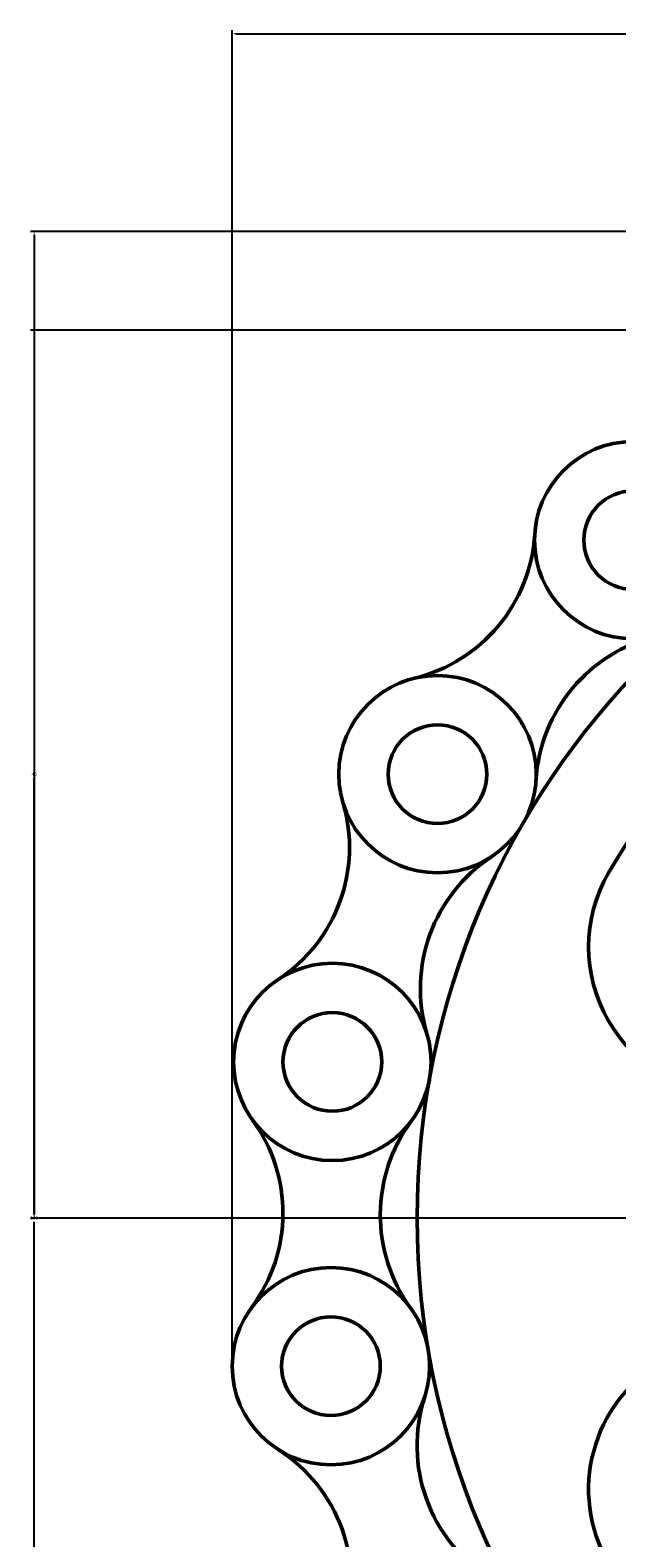
# Model space of a CAD drawing. Units: inches. Extents: x 413 to 622, y 326 to 447.
# Tile 2 of 15: x 413 to 443, y 370 to 447. Entities that reach past the tile are written whole.
import ezdxf

# ---------------------------------------------------------------- set-up
doc = ezdxf.new("R2010")
doc.units = ezdxf.units.IN
doc.header["$MEASUREMENT"] = 0
doc.layers.add('M-DIMS', color=2, linetype='Continuous', lineweight=18)
doc.layers.add('M-OUTL', color=7, linetype='Continuous', lineweight=50)
doc.styles.get("Standard").update_dxf_attribs({"font": 'arial.ttf'})
doc.dimstyles.get("Standard").update_dxf_attribs({"dimtxt": 0.18, "dimasz": 0.18, "dimexe": 0.18, "dimexo": 0.0625, "dimgap": 0.09, "dimtad": 0, "dimtih": 1, "dimtoh": 1, "dimdec": 4, "dimzin": 0, "dimdsep": 46, "dimtxsty": 'Standard', "dimcen": 0.09, "dimadec": 0, "dimazin": 0, "dimtfac": 1, "dimtdec": 4, "dimtofl": 0, "dimtmove": 0, "dimatfit": 3, "dimfxl": 1, "dimtolj": 1, "dimtzin": 0, "dimarcsym": 0})

# ---------------------------------------------------------------- blocks, each defined once
blk = doc.blocks.new('CHAIN-ROLLER-PIN')
for radius in [5, 2.5]:
    blk.add_circle((5, 5), radius)
blk = doc.blocks.new('SPROCKET-WEB-SLOT')
for centre, radius, start, end in [((7.501, 21.25), 7.5, 30, 210), ((31.317, 35), 20, 210, 270), ((31.317, 35), 35, 210, 270), ((31.317, 7.5), 7.5, 270, 90)]:
    blk.add_arc(centre, radius, start, end)
blk = doc.blocks.new('*D10')
at = {"layer": 'Defpoints', "color": 0, "transparency": 16777216}
for p in [(413.283, 436.392), (472.684, 436.392), (472.684, 336.392)]:
    blk.add_point(p, dxfattribs=at)
at = {"layer": 'M-DIMS', "color": 0, "lineweight": -2, "transparency": 16777216}
for p, q in [((472.621, 436.392), (413.103, 436.392)), ((413.283, 436.212), (413.283, 386.573)), ((413.283, 336.572), (413.283, 386.21)), ((472.621, 336.392), (413.103, 336.392))]:
    blk.add_line(p, q, dxfattribs=at)
at = {"layer": 'M-DIMS', "color": 0, "transparency": 16777216}
for points in [[(413.253, 436.212), (413.313, 436.212), (413.283, 436.392)], [(413.253, 336.572), (413.313, 336.572), (413.283, 336.392)]]:
    blk.add_solid(points, dxfattribs=at)
at = {"layer": 'M-DIMS', "color": 0, "transparency": 16777216, "insert": (413.283, 386.392), "char_height": 0.18, "attachment_point": 5}
blk.add_mtext('\\A1;100', dxfattribs=at)
blk = doc.blocks.new('*D11')
at = {"layer": 'Defpoints', "color": 0, "transparency": 16777216}
for p in [(621.66, 446.422), (621.66, 388.074), (423.314, 378.888)]:
    blk.add_point(p, dxfattribs=at)
at = {"layer": 'M-DIMS', "color": 0, "lineweight": -2, "transparency": 16777216}
for p, q in [((423.314, 378.95), (423.314, 446.602)), ((423.494, 446.422), (522.031, 446.422)), ((621.48, 446.422), (522.943, 446.422)), ((621.66, 388.137), (621.66, 446.602))]:
    blk.add_line(p, q, dxfattribs=at)
at = {"layer": 'M-DIMS', "color": 0, "transparency": 16777216}
for points in [[(423.494, 446.452), (423.494, 446.392), (423.314, 446.422)], [(621.48, 446.452), (621.48, 446.392), (621.66, 446.422)]]:
    blk.add_solid(points, dxfattribs=at)
at = {"layer": 'M-DIMS', "color": 0, "transparency": 16777216, "insert": (522.487, 446.422), "char_height": 0.18, "attachment_point": 5}
blk.add_mtext('\\A1;198.35', dxfattribs=at)
blk = doc.blocks.new('*D13')
at = {"layer": 'Defpoints', "color": 0, "transparency": 16777216}
for p in [(413.283, 431.392), (472.684, 431.392), (472.684, 386.392)]:
    blk.add_point(p, dxfattribs=at)
at = {"layer": 'M-DIMS', "color": 0, "lineweight": -2, "transparency": 16777216}
for p, q in [((472.621, 431.392), (413.103, 431.392)), ((413.283, 431.212), (413.283, 409.073)), ((413.283, 386.572), (413.283, 408.71)), ((472.621, 386.392), (413.103, 386.392))]:
    blk.add_line(p, q, dxfattribs=at)
at = {"layer": 'M-DIMS', "color": 0, "transparency": 16777216}
for points in [[(413.253, 431.212), (413.313, 431.212), (413.283, 431.392)], [(413.253, 386.572), (413.313, 386.572), (413.283, 386.392)]]:
    blk.add_solid(points, dxfattribs=at)
at = {"layer": 'M-DIMS', "color": 0, "transparency": 16777216, "insert": (413.283, 408.892), "char_height": 0.18, "attachment_point": 5}
blk.add_mtext('\\A1;45', dxfattribs=at)
blk = doc.blocks.new('*D24')
at = {"layer": 'Defpoints', "color": 0, "transparency": 16777216}
for p in [(432.684, 386.391), (512.684, 386.392)]:
    blk.add_point(p, dxfattribs=at)
at = {"layer": 'M-DIMS', "color": 0, "lineweight": -2, "transparency": 16777216}
for p, q in [((472.594, 386.392), (472.774, 386.392)), ((472.684, 386.302), (472.684, 386.482)), ((536.684, 386.392), (512.864, 386.392))]:
    blk.add_line(p, q, dxfattribs=at)
at = {"layer": 'M-DIMS', "color": 0, "transparency": 16777216}
blk.add_solid([(512.864, 386.422), (512.864, 386.362), (512.684, 386.392)], dxfattribs=at)
at = {"layer": 'M-DIMS', "color": 0, "transparency": 16777216, "insert": (537, 386.392), "char_height": 0.18, "attachment_point": 5}
blk.add_mtext('\\A1;∅80', dxfattribs=at)

msp = doc.modelspace()

# ---------------------------------------------------------------- linework, layer by layer
at = {"layer": 'M-OUTL'}
msp.add_circle((472.6836, 386.3915), 40, dxfattribs=at)
for centre, start, end in [((430.6487, 421.5253), 283.63116, 356.589334), ((446.6894, 408.1181), 103.63116, 176.589334), ((421.254, 405.1783), 303.269816, 16.596479), ((440.844, 398.0222), 123.269816, 196.596479), ((417.8834, 386.6473), 323.352902, 36.112297), ((438.8159, 386.5496), 143.352902, 216.112297), ((440.6768, 374.8687), 161.991387, 237.607516), ((421.3493, 367.9106), 341.991387, 57.607516)]:
    msp.add_arc(centre, 8, start, end, dxfattribs=at)

# ---------------------------------------------------------------- block references
at = {"layer": 'M-OUTL', "rotation": 239.9999999999996}
msp.add_blockref('SPROCKET-WEB-SLOT', (458.0314, 431.0122), dxfattribs=at)
at = {"layer": 'M-OUTL'}
for name, p in [('CHAIN-ROLLER-PIN', (438.6261, 415.7524)), ('CHAIN-ROLLER-PIN', (428.7129, 403.892)), ('CHAIN-ROLLER-PIN', (423.386, 389.3096)), ('CHAIN-ROLLER-PIN', (423.314, 373.8883)), ('SPROCKET-WEB-SLOT', (441.367, 351.392))]:
    msp.add_blockref(name, p, dxfattribs=at)

# ---------------------------------------------------------------- dimensions: what is measured, and where the dimension line sits
at = {"layer": 'M-DIMS'}
dim = msp.add_linear_dim(base=(621.66, 446.422), p1=(423.3136, 378.8878), p2=(621.66, 388.0741), dimstyle='Standard', override={"dimdec": 2, "dimlfac": 1, "dimrnd": 0, "dimzin": 0, "dimdsep": 46, "dimlunit": 2}, dxfattribs=at)
dim.commit()
dim.dimension.update_dxf_attribs({"geometry": '*D11', "text_midpoint": (522.4868, 446.422)})
for base, p1, p2, picture, middle in [((413.2831, 436.3915), (472.6836, 336.3915), (472.6836, 436.3915), '*D10', (413.2831, 386.3915)), ((413.2831, 431.3915), (472.6836, 386.3915), (472.6836, 431.3915), '*D13', (413.2831, 408.8915))]:
    dim = msp.add_linear_dim(base=base, p1=p1, p2=p2, angle=90, dimstyle='Standard', override={"dimdec": 0, "dimlfac": 1, "dimrnd": 0, "dimzin": 0, "dimdsep": 46, "dimlunit": 2}, dxfattribs=at)
    dim.commit()
    dim.dimension.update_dxf_attribs({"geometry": picture, "text_midpoint": middle})
dim = msp.add_diameter_dim_2p(p1=(432.6836, 386.391), p2=(512.6836, 386.392), dimstyle='Standard', override={"dimdec": 0, "dimlfac": 1, "dimrnd": 0, "dimzin": 0, "dimdsep": 46, "dimlunit": 2}, dxfattribs=at)
dim.commit()
dim.dimension.update_dxf_attribs({"geometry": '*D24', "text_midpoint": (536.6836, 386.3923), "dimtype": 163})

doc.saveas('drawing.dxf')
